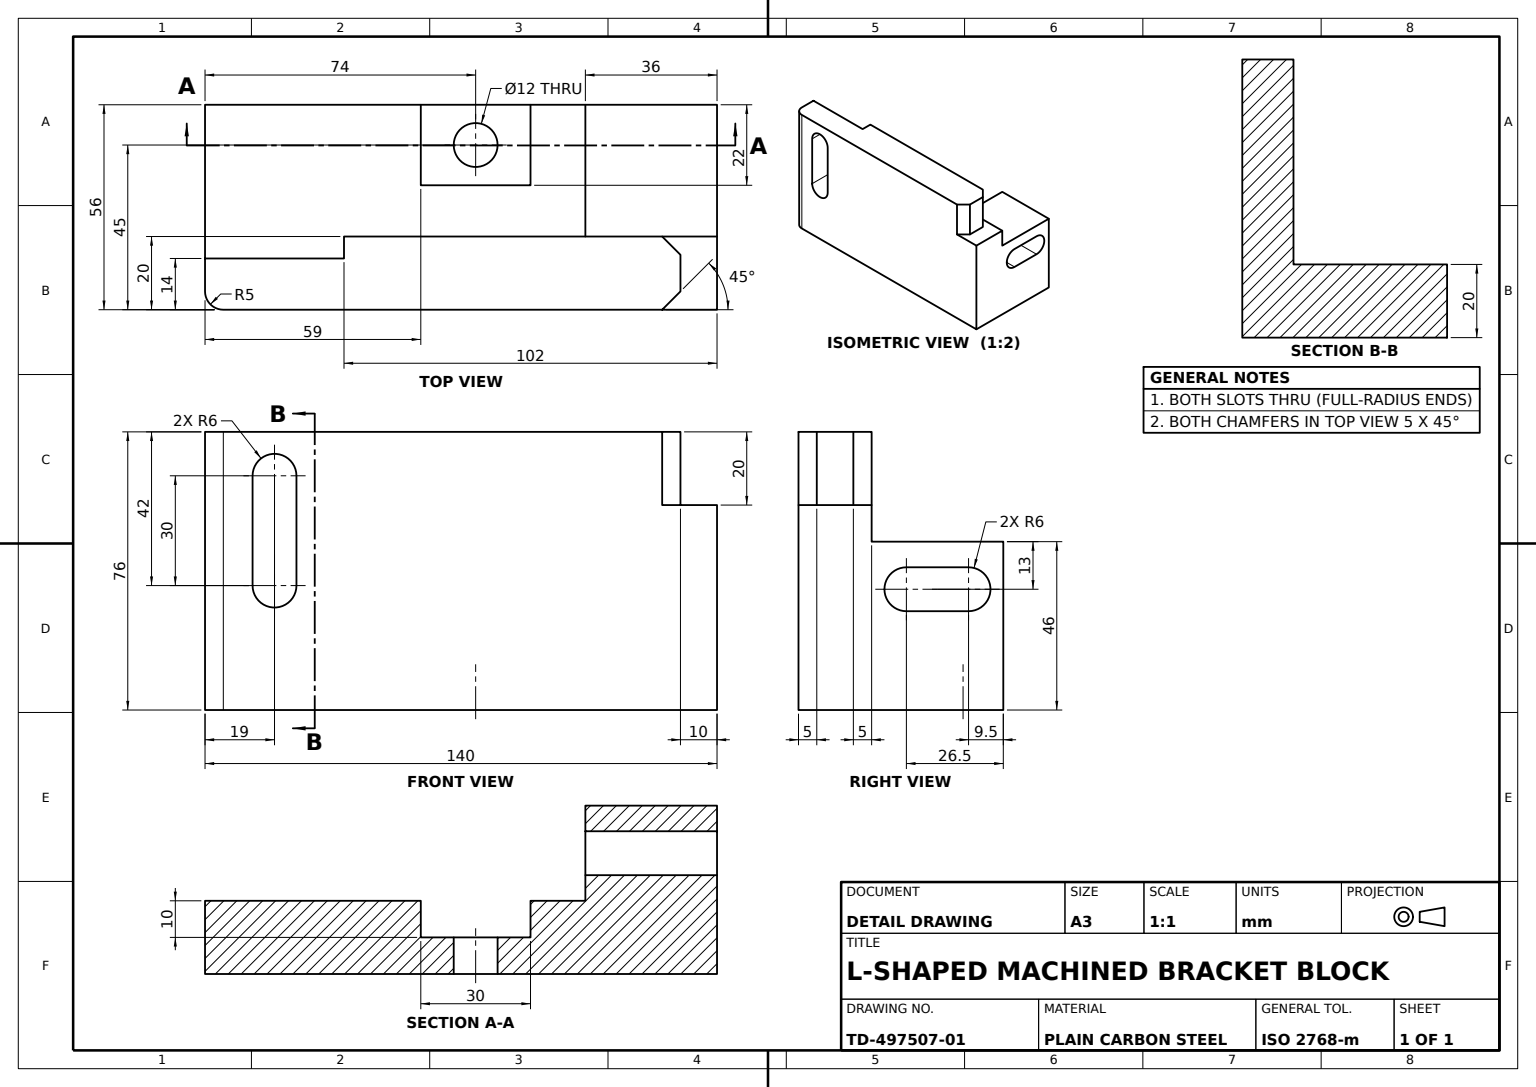
SolidWorks part; units mm, degrees
material "Plain Carbon Steel"
ref_plane "Front Plane" through (0, 0, 0) normal (0, 0, 1) x (1, 0, 0)
ref_plane "Top Plane" through (0, 0, 0) normal (0, 1, 0) x (1, 0, 0)
ref_plane "Right Plane" through (0, 0, 0) normal (1, 0, 0) x (0, 0, -1)
sketch "Base Plate Sketch" plane through (0, 0, 0) normal (0, 1, 0) x (1, 0, 0)
  line L1 (28, 0) -> (28, 70)
  line L2 (28, 70) -> (-28, 70)
  line L3 (-28, 70) -> (-28, -70)
  line L4 (-28, -70) -> (28, -70)
  line L5 (28, -70) -> (28, 0)
  dimension "D1" = 140
  dimension "D2" = 56
  dimension "D3" = 28
  dimension "D4" = 70
extrude "Base Plate" add sketch "Base Plate Sketch" along normal blind 20
sketch "Upright Wall Sketch" plane through (0, 20, 0) normal (0, 1, 0) x (1, 0, 0)
  line L0 (28, -70) -> (8, -70)
  line L1 (-28, -70) -> (28, -70) construction
  line L2 (8, -70) -> (8, 70)
  line L3 (28, 70) -> (-28, 70) construction
  line L4 (8, 70) -> (28, 70)
  line L5 (28, 70) -> (28, -70)
  dimension "D1" = 20
extrude "Upright Wall" add sketch "Upright Wall Sketch" along normal blind 56
sketch "Wall Profile Cut Sketch" plane through (0, 76, 0) normal (0, 1, 0) x (1, 0, 0)
  line L0 (28, -70) -> (28, -32)
  line L1 (28, -70) -> (28, 70) construction
  line L2 (28, -32) -> (14, -32)
  line L3 (14, -32) -> (14, -70)
  line L4 (8, -70) -> (28, -70) construction
  line L5 (14, -70) -> (28, -70)
  line L6 (14, -32) -> (8, -32)
  line L7 (8, 70) -> (8, -70) construction
  line L8 (8, -32) -> (8, -70)
  line L9 (8, -70) -> (14, -70)
  line M3 (8, 70) -> (8, -70)
  line M4 (8, -70) -> (28, -70)
  dimension "D1" = 14
  dimension "D2" = 102
extrude "Wall Profile Cut" cut sketch "Wall Profile Cut Sketch" against normal blind 56 contours L3 L6 M3 M4
sketch "Wall Slot Sketch" plane through (14, 0, 0) normal (-1, 0, 0) x (0, 0, 1)
  line L0 (32, 76) -> (70, 76) construction
  line L1 (32, 20) -> (32, 76) construction
  line L2 (57, 64) -> (57, 34)
  line L4 (45, 34) -> (45, 64)
  arc A0 (57, 64) -> (45, 64) centre (51, 64) ccw
  arc A1 (45, 34) -> (57, 34) centre (51, 34) ccw
  dimension "D1" = 6
  dimension "D2" = 19
  dimension "D3" = 12
  dimension "D4" = 42
extrude "Wall Slot" cut sketch "Wall Slot Sketch" against normal blind 56
sketch "Top Ridge Sketch" plane through (-28, 0, 0) normal (-1, 0, 0) x (0, 0, 1)
  line L0 (-70, 0) -> (-70, 46)
  line L1 (-70, 76) -> (-70, 20) construction
  line L2 (-70, 46) -> (-34, 46)
  line L3 (-34, 46) -> (-34, 0)
  line L4 (-70, 0) -> (70, 0) construction
  line L5 (-34, 0) -> (-70, 0)
  dimension "D1" = 104
  dimension "D2" = 46
extrude "Top Ridge" add sketch "Top Ridge Sketch" against normal blind 36
sketch "Wall Notch Sketch" plane through (-28, 0, 0) normal (-1, 0, 0) x (0, 0, 1)
  line L0 (-34, 20) -> (-34, 46) construction
  line L1 (-34, 20) -> (70, 20) construction
  line L2 (-19, 20) -> (-19, 10)
  line L3 (-19, 10) -> (11, 10)
  line L4 (11, 10) -> (11, 20)
  line L5 (-34, 20) -> (32, 20) construction
  line L6 (11, 20) -> (-19, 20)
  dimension "D1" = 15
  dimension "D2" = 45
  dimension "D3" = 10
extrude "Wall Notch" cut sketch "Wall Notch Sketch" against normal blind 22
sketch "Round Cut Sketch" plane through (0, 20, 0) normal (0, 1, 0) x (1, 0, 0)
  line L0 (-28, -11) -> (-28, -70) construction
  line L1 (-28, -70) -> (14, -70) construction
  circle A0 centre (-17, 4) radius 6
  dimension "D1" = 12
  dimension "D2" = 11
  dimension "D3" = 74
extrude "Round Cut" cut sketch "Round Cut Sketch" against normal blind 65
sketch "Step Cut Sketch" plane through (8, 0, 0) normal (-1, 0, 0) x (0, 0, 1)
  line L0 (-34, 46) -> (-70, 46) construction
  line L1 (-70, 76) -> (-70, 46) construction
  line L2 (-70, 56) -> (-60, 56)
  line L3 (-60, 56) -> (-60, 76)
  line L4 (-70, 76) -> (32, 76) construction
  line L5 (-60, 76) -> (-70, 76)
  line L6 (-70, 76) -> (-70, 56)
  dimension "D1" = 10
  dimension "D2" = 10
extrude "Step Cut" cut sketch "Step Cut Sketch" against normal blind 65
chamfer "Step Chamfer 5mm" distance 5 1 edges at (8, 66, -60)
chamfer "Base Edge Chamfer 5x45" distance 5 angle 45 1 edges at (28, 66, -60)
fillet "Corner Fillet R5" radius 5 1 edges at (28, 38, 70)
sketch "Ridge Slot Sketch" plane through (0, 0, -34) normal (0, 0, 1) x (1, 0, 0)
  line L0 (-28, 20) -> (-28, 46) construction
  line L1 (-28, 20) -> (8, 20) construction
  line L2 (-18.5, 39) -> (-1.5, 39)
  line L3 (-18.5, 27) -> (-1.5, 27)
  arc A0 (-18.5, 39) -> (-18.5, 27) centre (-18.5, 33) ccw
  arc A1 (-1.5, 27) -> (-1.5, 39) centre (-1.5, 33) ccw
  dimension "D1" = 6
  dimension "D2" = 9.5
  dimension "D3" = 26.5
  dimension "D4" = 13
extrude "Ridge Slot" cut sketch "Ridge Slot Sketch" against normal blind 65
